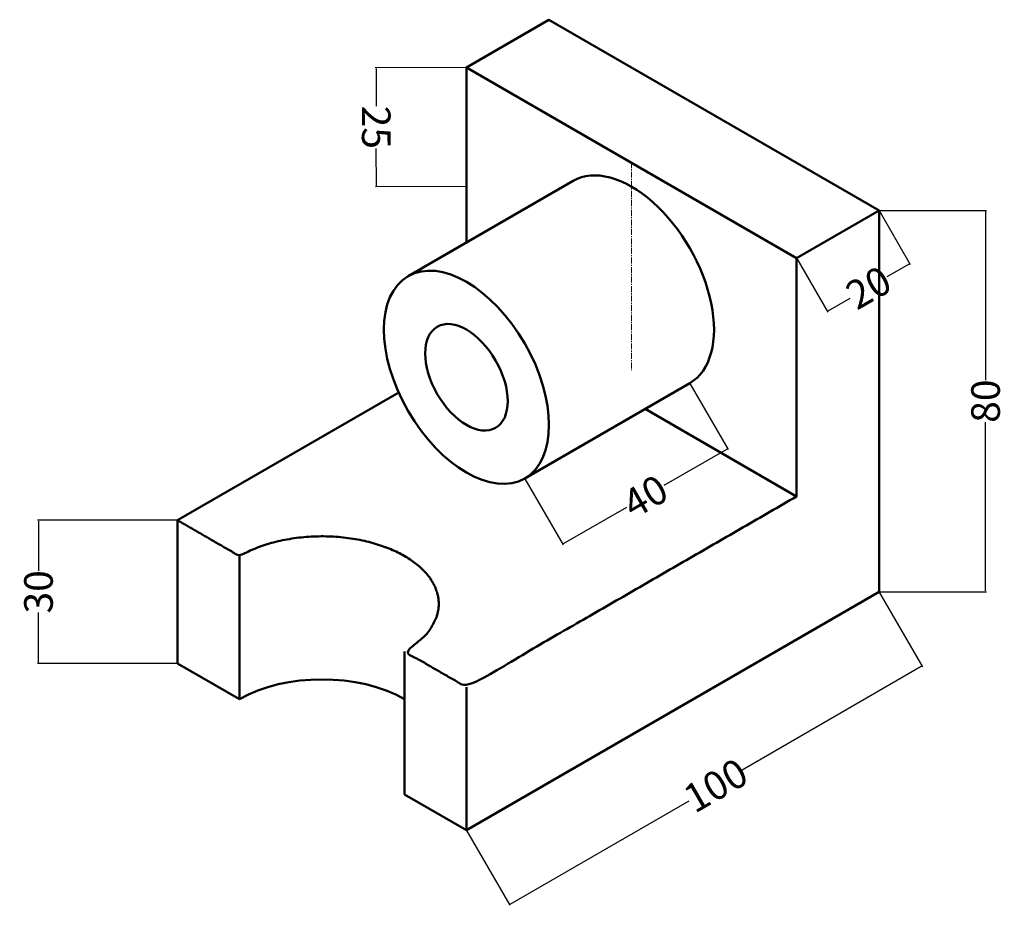
# Model space of a CAD drawing. Units: millimetres. Extents: x -32 to 174, y 12 to 198.
import ezdxf

# ---------------------------------------------------------------- set-up
doc = ezdxf.new("R2010")
doc.units = ezdxf.units.MM
doc.header["$MEASUREMENT"] = 0
doc.linetypes.add('CENTER', pattern=[2, 1.25, -0.25, 0.25, -0.25])
for name, color, linetype, lineweight in [('M-CNTR', 4, 'CENTER', 18), ('M-CONS', 8, 'Continuous', 13), ('M-DIMS', 2, 'Continuous', 25), ('M-OUTL', 7, 'Continuous', 50)]:
    doc.layers.add(name, color=color, linetype=linetype, lineweight=lineweight)
doc.styles.get("Standard").update_dxf_attribs({"font": 'arial.ttf'})
doc.dimstyles.get("Standard").update_dxf_attribs({"dimtxt": 6, "dimasz": 0.18, "dimexe": 0.18, "dimexo": 0.0625, "dimgap": 0.09, "dimtad": 0, "dimtoh": 1, "dimdec": 0, "dimzin": 0, "dimdsep": 46, "dimtxsty": 'Standard', "dimcen": 0.09, "dimadec": 0, "dimazin": 0, "dimtfac": 1, "dimtdec": 0, "dimtofl": 0, "dimtmove": 0, "dimatfit": 3, "dimfxl": 1, "dimtolj": 1, "dimtzin": 0, "dimarcsym": 0})

# ---------------------------------------------------------------- blocks, each defined once
blk = doc.blocks.new('*U1')
at = {"layer": 'M-CNTR', "color": 0, "transparency": 16777216}
blk.add_line((0, 21.8), (0, -21.8), dxfattribs=at)
blk = doc.blocks.new('*D2')
at = {"layer": 'Defpoints', "color": 0, "transparency": 16777216}
for p in [(61.46, 187.67), (42.61, 162.66), (61.52, 162.71)]:
    blk.add_point(p, dxfattribs=at)
at = {"layer": 'M-DIMS', "color": 0, "lineweight": -2, "transparency": 16777216}
for p, q in [((61.4, 187.67), (42.37, 187.63)), ((42.55, 187.45), (42.57, 179.61)), ((42.61, 162.84), (42.59, 170.68)), ((61.46, 162.71), (42.43, 162.66))]:
    blk.add_line(p, q, dxfattribs=at)
at = {"layer": 'M-DIMS', "color": 0, "transparency": 16777216}
for points in [[(42.58, 187.45), (42.52, 187.45), (42.55, 187.63)], [(42.64, 162.84), (42.58, 162.84), (42.61, 162.66)]]:
    blk.add_solid(points, dxfattribs=at)
at = {"layer": 'M-DIMS', "color": 0, "transparency": 16777216, "insert": (42.58, 175.14), "char_height": 6, "attachment_point": 5, "rotation": 270.1481}
blk.add_mtext('\\A1;25', dxfattribs=at)
blk = doc.blocks.new('*D3')
at = {"layer": 'Defpoints', "color": 0, "transparency": 16777216}
for p in [(108.41, 121.5), (116.36, 107.73), (73.77, 101.5)]:
    blk.add_point(p, dxfattribs=at)
at = {"layer": 'M-DIMS', "color": 0, "lineweight": -2, "transparency": 16777216}
for p, q in [((108.44, 121.44), (116.45, 107.57)), ((116.21, 107.64), (102.94, 99.98)), ((73.8, 101.44), (81.81, 87.57)), ((81.88, 87.82), (95.15, 95.48))]:
    blk.add_line(p, q, dxfattribs=at)
at = {"layer": 'M-DIMS', "color": 0, "transparency": 16777216}
for points in [[(116.19, 107.67), (116.22, 107.61), (116.36, 107.73)], [(81.86, 87.85), (81.89, 87.79), (81.72, 87.73)]]:
    blk.add_solid(points, dxfattribs=at)
at = {"layer": 'M-DIMS', "color": 0, "transparency": 16777216, "insert": (99.04, 97.73), "char_height": 6, "attachment_point": 5, "rotation": 30}
blk.add_mtext('\\A1;40', dxfattribs=at)
blk = doc.blocks.new('*D4')
at = {"layer": 'Defpoints', "color": 0, "transparency": 16777216}
for p in [(148.13, 77.71), (157.13, 62.12), (61.52, 27.71)]:
    blk.add_point(p, dxfattribs=at)
at = {"layer": 'M-DIMS', "color": 0, "lineweight": -2, "transparency": 16777216}
for p, q in [((148.16, 77.66), (157.22, 61.96)), ((156.97, 62.03), (119.39, 40.33)), ((70.68, 12.21), (108.26, 33.9)), ((61.56, 27.66), (70.62, 11.96))]:
    blk.add_line(p, q, dxfattribs=at)
at = {"layer": 'M-DIMS', "color": 0, "transparency": 16777216}
for points in [[(156.96, 62.05), (156.99, 62), (157.13, 62.12)], [(70.67, 12.23), (70.7, 12.18), (70.53, 12.12)]]:
    blk.add_solid(points, dxfattribs=at)
at = {"layer": 'M-DIMS', "color": 0, "transparency": 16777216, "insert": (113.83, 37.12), "char_height": 6, "attachment_point": 5, "rotation": 30}
blk.add_mtext('\\A1;100', dxfattribs=at)
blk = doc.blocks.new('*D5')
at = {"layer": 'Defpoints', "color": 0, "transparency": 16777216}
for p in [(0.9, 92.71), (-28.31, 62.71), (0.9, 62.71)]:
    blk.add_point(p, dxfattribs=at)
at = {"layer": 'M-DIMS', "color": 0, "lineweight": -2, "transparency": 16777216}
for p, q in [((0.84, 92.71), (-28.49, 92.71)), ((-28.31, 92.53), (-28.31, 82.09)), ((-28.31, 62.89), (-28.31, 73.34)), ((0.84, 62.71), (-28.49, 62.71))]:
    blk.add_line(p, q, dxfattribs=at)
at = {"layer": 'M-DIMS', "color": 0, "transparency": 16777216}
for points in [[(-28.34, 92.53), (-28.28, 92.53), (-28.31, 92.71)], [(-28.34, 62.89), (-28.28, 62.89), (-28.31, 62.71)]]:
    blk.add_solid(points, dxfattribs=at)
at = {"layer": 'M-DIMS', "color": 0, "transparency": 16777216, "insert": (-28.31, 77.71), "char_height": 6, "attachment_point": 5, "rotation": 90}
blk.add_mtext('\\A1;30', dxfattribs=at)
blk = doc.blocks.new('*D6')
at = {"layer": 'Defpoints', "color": 0, "transparency": 16777216}
for p in [(148.13, 157.71), (130.81, 147.71), (154.58, 146.53)]:
    blk.add_point(p, dxfattribs=at)
at = {"layer": 'M-DIMS', "color": 0, "lineweight": -2, "transparency": 16777216}
for p, q in [((148.16, 157.66), (154.67, 146.38)), ((130.84, 147.66), (137.35, 136.38)), ((154.42, 146.44), (149.76, 143.75)), ((137.42, 136.62), (142.09, 139.32))]:
    blk.add_line(p, q, dxfattribs=at)
at = {"layer": 'M-DIMS', "color": 0, "transparency": 16777216}
for points in [[(154.41, 146.47), (154.44, 146.42), (154.58, 146.53)], [(137.4, 136.65), (137.43, 136.6), (137.26, 136.53)]]:
    blk.add_solid(points, dxfattribs=at)
at = {"layer": 'M-DIMS', "color": 0, "transparency": 16777216, "insert": (145.92, 141.53), "char_height": 6, "attachment_point": 5, "rotation": 30}
blk.add_mtext('\\A1;20', dxfattribs=at)
blk = doc.blocks.new('*D7')
at = {"layer": 'Defpoints', "color": 0, "transparency": 16777216}
for p in [(148.13, 157.71), (148.13, 77.71), (170.48, 77.71)]:
    blk.add_point(p, dxfattribs=at)
at = {"layer": 'M-DIMS', "color": 0, "lineweight": -2, "transparency": 16777216}
for p, q in [((148.19, 157.71), (170.66, 157.71)), ((170.48, 157.53), (170.48, 122.09)), ((170.48, 77.89), (170.48, 113.33)), ((148.19, 77.71), (170.66, 77.71))]:
    blk.add_line(p, q, dxfattribs=at)
at = {"layer": 'M-DIMS', "color": 0, "transparency": 16777216}
for points in [[(170.45, 157.53), (170.51, 157.53), (170.48, 157.71)], [(170.45, 77.89), (170.51, 77.89), (170.48, 77.71)]]:
    blk.add_solid(points, dxfattribs=at)
at = {"layer": 'M-DIMS', "color": 0, "transparency": 16777216, "insert": (170.48, 117.71), "char_height": 6, "attachment_point": 5, "rotation": 90}
blk.add_mtext('\\A1;80', dxfattribs=at)

msp = doc.modelspace()

# ---------------------------------------------------------------- linework, layer by layer
at = {"layer": 'M-CONS'}
msp.add_line((13.89, 85.21), (13.89, 85.21), dxfattribs=at)
at = {"layer": 'M-OUTL'}
for p, q in [((49.28, 143.92), (83.92, 163.92)), ((73.77, 101.5), (108.41, 121.5)), ((0.9, 92.71), (47.3, 119.5)), ((0.9, 62.71), (0.9, 92.71)), ((13.89, 55.21), (13.89, 85.21)), ((48.53, 35.21), (48.53, 65.21)), ((13.89, 55.21), (0.9, 62.71)), ((61.52, 27.71), (48.53, 35.21))]:
    msp.add_line(p, q, dxfattribs=at)
for points in [[(130.81, 147.71), (148.13, 157.71), (78.84, 197.71), (61.52, 187.71), (61.52, 151)], [(99.01, 116.07), (130.81, 97.71), (130.81, 147.71), (61.52, 187.71)], [(148.13, 157.71), (148.13, 77.71), (61.52, 27.71), (61.52, 57.71)]]:
    msp.add_lwpolyline(points, dxfattribs=at)
for centre, major_axis, start_param, end_param in [((96.16, 142.71), (12.25, -21.21), 0, 3.141593), ((31.21, 45.21), (-24.49, 0), 3.926991, 5.497787)]:
    msp.add_ellipse(centre, major_axis=major_axis, ratio=0.57735, start_param=start_param, end_param=end_param, dxfattribs=at)
for major_axis in [(12.25, -21.21), (6.12, -10.61)]:
    msp.add_ellipse((61.52, 122.71), major_axis=major_axis, ratio=0.57735, dxfattribs=at)
msp.add_rational_spline([(130.81, 97.71), (96.16, 77.71), (61.52, 57.71), (55.03, 61.46), (48.53, 65.21), (65.85, 75.21), (48.53, 85.21), (31.21, 95.21), (13.89, 85.21), (7.4, 88.96), (0.9, 92.71)], [1, 1, 1, 1, 1, 0.707106781187, 1, 0.707106781187, 1, 1, 1], degree=2, knots=[0, 0, 0, 1, 1, 2, 2, 3.570796, 3.570796, 5.141593, 5.141593, 6.141593, 6.141593, 6.141593], dxfattribs=at)

# ---------------------------------------------------------------- block references
at = {"layer": 'M-CNTR'}
msp.add_blockref('*U1', (96.16, 146.03), dxfattribs=at)

# ---------------------------------------------------------------- dimensions: what is measured, and where the dimension line sits
at = {"layer": 'M-DIMS'}
for p1, p2, distance, picture, middle in [((61.46, 187.67), (61.52, 162.71), -18.91, '*D2', (42.58, 175.14)), ((130.81, 147.71), (148.13, 157.71), -12.91, '*D6', (145.92, 141.53)), ((148.13, 157.71), (148.13, 77.71), 22.35, '*D7', (170.48, 117.71)), ((73.77, 101.5), (108.41, 121.5), -15.9, '*D3', (99.04, 97.73)), ((0.9, 92.71), (0.9, 62.71), -29.22, '*D5', (-28.31, 77.71)), ((61.52, 27.71), (148.13, 77.71), -18.01, '*D4', (113.83, 37.12))]:
    dim = msp.add_aligned_dim(p1=p1, p2=p2, distance=distance, dimstyle='Standard', override={"dimclrd": 0, "dimclre": 0, "dimclrt": 0}, dxfattribs=at)
    dim.commit()
    dim.dimension.update_dxf_attribs({"geometry": picture, "text_midpoint": middle})

doc.saveas('drawing.dxf')
